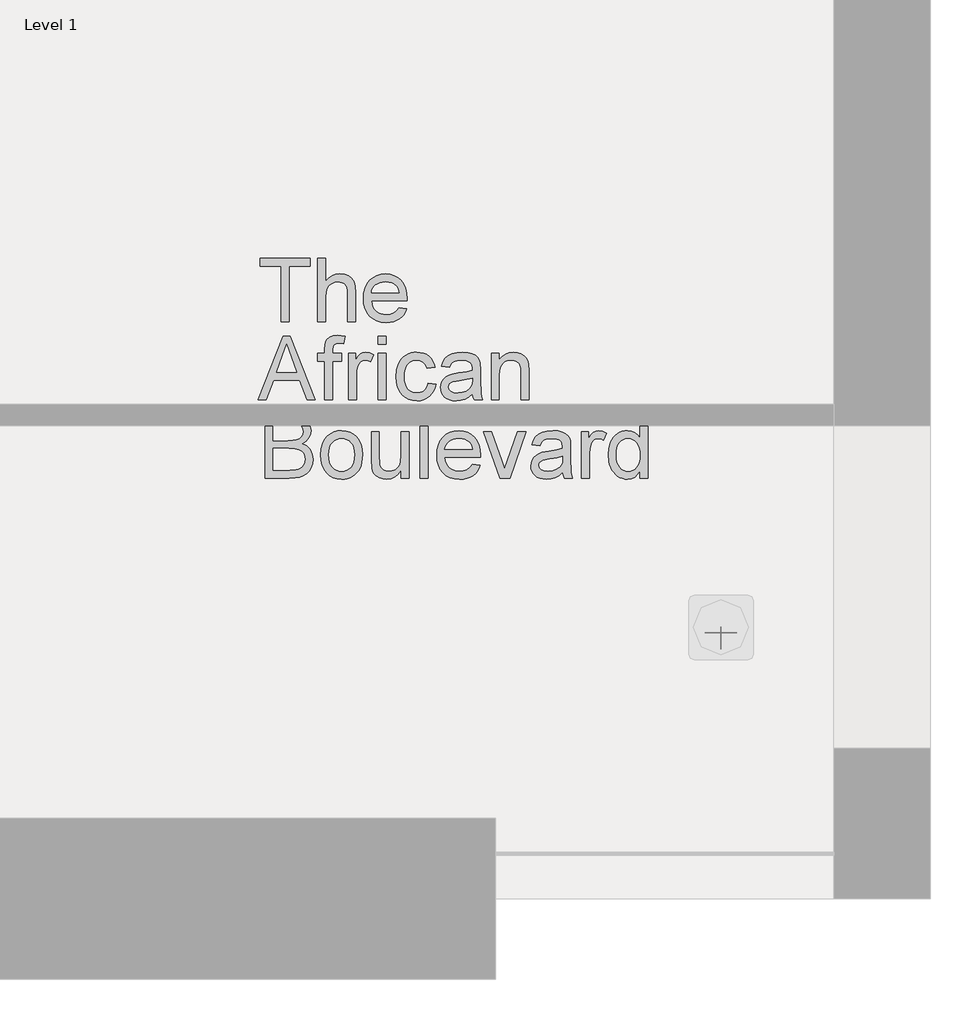
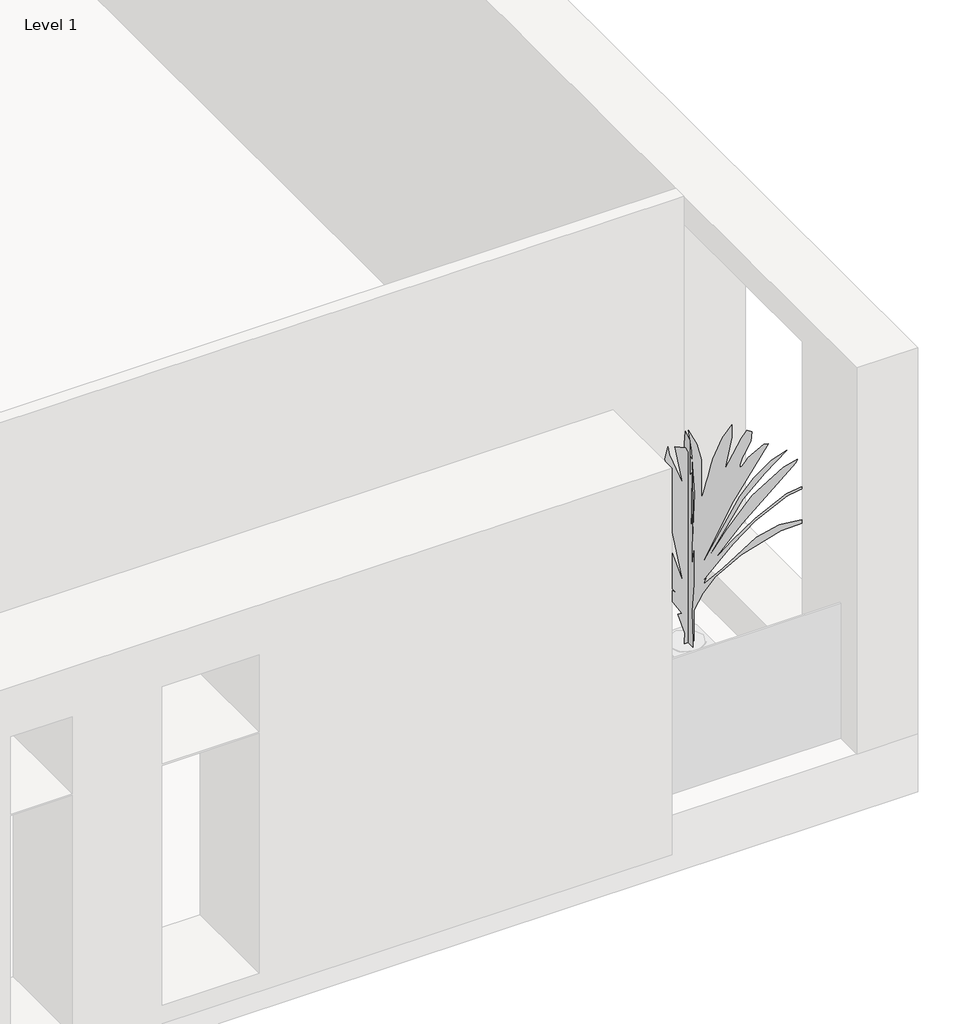
# One storey, part 3 of 3: 1 geographic element, 1 proxy.
"""IFC4 building model written with IfcOpenShell, lengths in millimetres."""

from ifc_helpers import new_model, si_unit, origin, origin_with_axes, place, context, project, spatial, polyline, outline, extrude, transform, mapped, element, save
from components import rpc_tree_tropical_0177ab4a

model = new_model("IFC4")

# Units and contexts
model_context = context("Model", 3, world=origin())
ifc_project = project(units=[si_unit("LENGTHUNIT", "METRE", prefix="MILLI")], contexts=[model_context])

# Site, building, storey
site = spatial("IfcSite", under=ifc_project)
building = spatial("IfcBuilding", under=site)
storey = spatial("IfcBuildingStorey", under=building, Name="Level 1", Elevation=0.0)

# Proxy
placement = place(None, origin())
element("IfcBuildingElementProxy", 1, Name="24\" Arial", ObjectType="24\" Arial", at=placement, inside=storey, context=model_context, shape_type="SweptSolid", body=[
    extrude(outline(polyline([(215.7046154, 0.0), (215.7046154, 525.1938462), (18.7569231, 525.1938462), (18.7569231, 600.2215385), (487.68, 600.2215385), (487.68, 525.1938462), (290.7323077, 525.1938462), (290.7323077, 0.0), (215.7046154, 0.0)])), origin_with_axes(), (0.0, 0.0, 1.0), 152.4),
    extrude(outline(polyline([(562.7076923, 0.0), (562.7076923, 600.2215385), (637.7353846, 600.2215385), (637.7353846, 379.5346154), (665.293774, 410.4359135), (696.2408654, 432.5082692), (730.5766587, 445.7516827), (768.3011538, 450.1661538), (813.6181731, 445.3487019), (852.5607692, 430.8963462), (883.2239423, 407.9447596), (903.7026923, 377.6296154), (915.2425962, 335.9760577), (919.0892308, 279.0092308), (919.0892308, 0.0), (844.0615385, 0.0), (844.0615385, 271.2426923), (842.5686779, 296.5755288), (838.0900962, 318.2082692), (830.6257933, 336.1409135), (820.1757692, 350.3734615), (806.9873077, 361.208149), (791.3076923, 368.9472115), (773.1369231, 373.590649), (752.475, 375.1384615), (720.7677404, 370.9621154), (691.0021154, 358.4330769), (666.3470192, 338.7602885), (649.9713462, 313.1526923), (640.794375, 279.1191346), (637.7353846, 234.1684615), (637.7353846, 0.0), (562.7076923, 0.0)])), origin_with_axes(), (0.0, 0.0, 1.0), 152.4),
    extrude(outline(polyline([(1330.8623077, 131.2984615), (1404.4246154, 121.92), (1393.1457332, 92.4566106), (1377.9194712, 66.4918269), (1358.7458293, 44.025649), (1335.6248077, 25.0580769), (1308.7945313, 9.9920913), (1278.493125, -0.7693269), (1244.7205889, -7.2261779), (1207.4769231, -9.3784615), (1160.9234856, -5.6646274), (1119.4439423, 5.476875), (1083.0382933, 24.0460457), (1051.7065385, 50.0428846), (1026.5110817, 82.7438582), (1008.5143269, 121.4254327), (997.716274, 166.0876082), (994.1169231, 216.7303846), (997.7529087, 269.0904087), (1008.6608654, 315.2408654), (1026.8407933, 355.1817548), (1052.2926923, 388.9130769), (1083.5420192, 415.7112981), (1119.1142308, 434.8528846), (1159.0093269, 446.3378365), (1203.2273077, 450.1661538), (1246.0211178, 446.3469952), (1284.7210096, 434.8895192), (1319.3269832, 415.793726), (1349.8390385, 389.0596154), (1374.7459976, 355.4015625), (1392.5366827, 315.5339423), (1403.2110938, 269.4567548), (1406.7692308, 217.17), (1406.3296154, 196.9476923), (1069.1446154, 196.9476923), (1073.4903966, 167.0080529), (1082.1315865, 140.7868269), (1095.0681851, 118.2840144), (1112.3001923, 99.4996154), (1132.8751082, 84.6900721), (1155.8404327, 74.1118269), (1181.1961659, 67.7648798), (1208.9423077, 65.6492308), (1248.8740385, 69.5691346), (1282.5046154, 81.3288462), (1309.8340385, 101.6610577), (1330.8623077, 131.2984615)]), holes=[polyline([(1069.1446154, 271.9753846), (1331.7415385, 271.9753846), (1321.59375, 311.6140385), (1312.8655529, 327.2020673), (1301.7011538, 339.9692308), (1281.2407212, 355.3557692), (1257.9594231, 366.3461538), (1231.8572596, 372.9403846), (1202.9342308, 375.1384615), (1176.5527284, 373.3845793), (1152.3601442, 368.1229327), (1130.3564784, 359.3535216), (1110.5417308, 347.0763462), (1093.9141947, 331.8592428), (1081.4721635, 314.2700481), (1073.215637, 294.308762), (1069.1446154, 271.9753846)])]), origin_with_axes(), (0.0, 0.0, 1.0), 152.4),
    extrude(outline(polyline([(-4.1030769, -740.8984615), (235.4873077, -140.6769231), (299.3780769, -140.6769231), (538.8219231, -740.8984615), (459.5446154, -740.8984615), (390.9646154, -553.3292308), (143.6076923, -553.3292308), (75.0276923, -740.8984615), (-4.1030769, -740.8984615)]), holes=[polyline([(171.1569231, -478.3015385), (363.5619231, -478.3015385), (309.3426923, -330.7373077), (267.2861538, -215.7046154), (229.9188462, -317.8419231), (171.1569231, -478.3015385)])]), origin_with_axes(), (0.0, 0.0, 1.0), 152.4),
    extrude(outline(polyline([(628.3569231, -740.8984615), (628.3569231, -375.1384615), (562.7076923, -375.1384615), (562.7076923, -300.1107692), (628.3569231, -300.1107692), (628.3569231, -255.7096154), (630.3351923, -218.9650962), (636.27, -193.1376923), (651.3634615, -168.1895192), (674.6630769, -148.4434615), (707.2678846, -135.5847115), (750.2769231, -131.2984615), (782.8450962, -133.35), (818.7103846, -139.5046154), (807.72, -209.8430769), (764.4911538, -206.3261538), (735.9711058, -209.4400962), (717.2325, -218.7819231), (706.8465865, -236.6229808), (703.3846154, -265.2346154), (703.3846154, -300.1107692), (787.7907692, -300.1107692), (787.7907692, -375.1384615), (703.3846154, -375.1384615), (703.3846154, -740.8984615), (628.3569231, -740.8984615)])), origin_with_axes(), (0.0, 0.0, 1.0), 152.4),
    extrude(outline(polyline([(853.44, -740.8984615), (853.44, -300.1107692), (919.0892308, -300.1107692), (919.0892308, -365.3203846), (943.3413462, -327.5134615), (965.6884615, -305.2396154), (988.1088462, -294.3591346), (1012.5807692, -290.7323077), (1049.9480769, -296.5205769), (1087.9015385, -313.8853846), (1062.8434615, -381.1465385), (1036.4665385, -369.6066346), (1010.0896154, -365.76), (987.6875481, -369.4600962), (967.6667308, -380.5603846), (951.4925481, -398.2182692), (940.6303846, -421.5911538), (931.5083654, -463.5011538), (928.4676923, -509.2211538), (928.4676923, -740.8984615), (853.44, -740.8984615)])), origin_with_axes(), (0.0, 0.0, 1.0), 152.4),
    extrude(outline(polyline([(1134.7938462, -740.8984615), (1134.7938462, -300.1107692), (1209.8215385, -300.1107692), (1209.8215385, -740.8984615), (1134.7938462, -740.8984615)])), origin_with_axes(), (0.0, 0.0, 1.0), 152.4),
    extrude(outline(polyline([(1134.7938462, -215.7046154), (1134.7938462, -140.6769231), (1209.8215385, -140.6769231), (1209.8215385, -215.7046154), (1134.7938462, -215.7046154)])), origin_with_axes(), (0.0, 0.0, 1.0), 152.4),
    extrude(outline(polyline([(1603.7169231, -581.4646154), (1678.7446154, -590.8430769), (1670.5842548, -626.2458534), (1657.82625, -657.5730288), (1640.470601, -684.8246034), (1618.5173077, -708.0005769), (1592.8913942, -726.4964784), (1564.5178846, -739.7078365), (1533.3967788, -747.6346514), (1499.5280769, -750.2769231), (1457.4486418, -746.5905649), (1419.7195673, -735.5314904), (1386.3408534, -717.0996995), (1357.3125, -691.2951923), (1333.8159736, -658.6033774), (1317.0327404, -619.5096635), (1306.9628005, -574.0140505), (1303.6061538, -522.1165385), (1309.3394712, -455.3499519), (1316.5061178, -425.304988), (1326.5394231, -397.4855769), (1339.5080769, -372.4503966), (1355.4807692, -350.758125), (1374.4575, -332.408762), (1396.4382692, -317.4023077), (1420.429363, -305.7341827), (1445.4370673, -297.3998077), (1471.4613822, -292.3991827), (1498.5023077, -290.7323077), (1531.7894351, -293.0219712), (1561.8985096, -299.8909615), (1588.8295313, -311.3392788), (1612.5825, -327.3669231), (1632.7544351, -347.6075481), (1648.9423558, -371.6948077), (1661.146262, -399.6287019), (1669.3661538, -431.4092308), (1594.3384615, -440.7876923), (1580.7287019, -408.0546635), (1559.5355769, -384.5901923), (1531.9313942, -370.4675481), (1499.0884615, -365.76), (1473.5953486, -368.0771394), (1450.6025481, -375.0285577), (1430.1100601, -386.6142548), (1412.1178846, -402.8342308), (1397.4686178, -424.0639904), (1387.0048558, -450.6790385), (1380.7265986, -482.679375), (1378.6338462, -520.065), (1380.6808053, -558.0138822), (1386.8216827, -590.3851442), (1397.0564784, -617.1787861), (1411.3851923, -638.3948077), (1429.0201803, -654.5186178), (1449.1737981, -666.035625), (1471.8460457, -672.9458293), (1497.0369231, -675.2492308), (1535.8879327, -669.4975962), (1552.6894832, -662.3080529), (1567.7417308, -652.2426923), (1580.6233774, -639.1916106), (1590.913125, -623.0449038), (1598.6109736, -603.8025721), (1603.7169231, -581.4646154)])), origin_with_axes(), (0.0, 0.0, 1.0), 152.4),
    extrude(outline(polyline([(2025.7476923, -684.6276923), (1989.9007212, -715.3641346), (1952.9913462, -735.4765385), (1914.1769712, -746.5768269), (1872.615, -750.2769231), (1839.2088101, -748.0513702), (1809.9148558, -741.3747115), (1784.733137, -730.2469471), (1763.6636538, -714.6680769), (1747.0269591, -695.6272356), (1735.1436058, -674.1135577), (1728.0135938, -650.1270433), (1725.6369231, -623.6676923), (1729.2271154, -592.5649038), (1739.9976923, -564.3196154), (1756.6114904, -540.1407692), (1777.7313462, -521.2373077), (1802.5512981, -506.9498077), (1830.2653846, -496.6188462), (1895.1819231, -485.3353846), (1971.8948077, -473.4657692), (2025.3080769, -459.5446154), (2025.7476923, -442.8392308), (2020.5822115, -409.3551923), (2014.1253606, -396.954375), (2005.0857692, -387.4476923), (1989.4611058, -377.9593269), (1970.4294231, -371.1819231), (1922.145, -365.76), (1877.4507692, -369.3685096), (1846.2380769, -380.1940385), (1824.9533654, -400.2148558), (1810.0430769, -431.4092308), (1735.0153846, -422.0307692), (1748.0389904, -381.0), (1767.4736538, -348.7615385), (1795.1327885, -324.1064423), (1832.8298077, -305.8257692), (1878.9344712, -294.5056731), (1931.8165385, -290.7323077), (1982.5371635, -294.0660577), (2022.7436538, -304.0673077), (2053.0587981, -319.1058173), (2074.1053846, -337.5513462), (2088.0631731, -360.3563942), (2097.1119231, -388.4734615), (2100.7753846, -454.1226923), (2100.7753846, -547.4676923), (2104.5853846, -677.8136538), (2110.2271154, -710.0337981), (2119.5323077, -740.8984615), (2044.5046154, -740.8984615), (2032.4884615, -714.8146154), (2025.7476923, -684.6276923)]), holes=[polyline([(2025.7476923, -534.5723077), (1975.3384615, -547.0647115), (1904.7069231, -557.5788462), (1840.1567308, -569.7415385), (1823.3597596, -578.0575962), (1810.9223077, -589.5242308), (1803.2290385, -603.2622115), (1800.6646154, -618.3923077), (1806.2513942, -640.7027885), (1823.0117308, -658.9834615), (1850.5792788, -671.1827885), (1888.5876923, -675.2492308), (1928.8857692, -670.7614904), (1964.4946154, -657.2982692), (1993.3626923, -637.460625), (2013.4384615, -613.8496154), (2022.3406731, -589.5242308), (2025.3080769, -555.8203846), (2025.7476923, -534.5723077)])]), origin_with_axes(), (0.0, 0.0, 1.0), 152.4),
    extrude(outline(polyline([(2203.9384615, -740.8984615), (2203.9384615, -300.1107692), (2278.9661538, -300.1107692), (2278.9661538, -361.6569231), (2305.0316827, -330.6274038), (2336.3359615, -308.4634615), (2372.8789904, -295.1650962), (2414.6607692, -290.7323077), (2451.6434135, -294.3041827), (2485.5121154, -305.0198077), (2513.7574038, -321.5420192), (2533.8698077, -342.5336538), (2547.5162019, -367.9397596), (2556.3634615, -397.7053846), (2560.32, -470.2419231), (2560.32, -740.8984615), (2485.2923077, -740.8984615), (2485.2923077, -480.3530769), (2483.1308654, -441.5570192), (2476.6465385, -413.9711538), (2464.6853365, -394.2067788), (2446.0932692, -378.8751923), (2422.2624519, -369.0387981), (2394.585, -365.76), (2371.8028486, -367.6008894), (2350.6417788, -373.1235577), (2331.1017909, -382.3280048), (2313.1828846, -395.2142308), (2298.2130649, -413.2476202), (2287.5203365, -437.8935577), (2281.1046995, -469.1520433), (2278.9661538, -507.0230769), (2278.9661538, -740.8984615), (2203.9384615, -740.8984615)])), origin_with_axes(), (0.0, 0.0, 1.0), 152.4),
    extrude(outline(polyline([(65.6492308, -1481.7969231), (65.6492308, -881.5753846), (294.6888462, -881.5753846), (357.6820673, -885.9898558), (406.8640385, -899.2332692), (426.8573798, -909.2482572), (444.5610577, -921.6353365), (459.9750721, -936.3945072), (473.0994231, -953.5257692), (491.0687019, -991.0396154), (497.0584615, -1030.3119231), (492.0212019, -1066.4519712), (476.9094231, -1100.4305769), (451.6132212, -1130.1595673), (416.0226923, -1153.5507692), (438.6674639, -1163.2039904), (458.5371635, -1175.7513462), (475.6317909, -1191.1928365), (489.9513462, -1209.5284615), (501.266863, -1230.1995433), (509.349375, -1252.6474038), (514.1988822, -1276.8720433), (515.8153846, -1302.8734615), (511.4009135, -1344.7285096), (498.1575, -1383.5428846), (478.393125, -1416.5506731), (454.4157692, -1440.9859615), (425.053125, -1458.6804808), (389.1328846, -1471.4659615), (345.4827404, -1479.2141827), (292.9303846, -1481.7969231), (65.6492308, -1481.7969231)]), holes=[polyline([(140.6769231, -1125.4153846), (277.6903846, -1125.4153846), (325.6084615, -1123.8034615), (357.7003846, -1118.9676923), (385.7075481, -1107.8490865), (405.8382692, -1091.1986538), (417.9826442, -1069.2728365), (422.0307692, -1042.3280769), (418.2574038, -1016.1709615), (406.9373077, -993.3842308), (388.5833654, -975.598125), (363.7084615, -964.4428846), (325.5351923, -958.5630288), (267.2861538, -956.6030769), (140.6769231, -956.6030769), (140.6769231, -1125.4153846)]), polyline([(140.6769231, -1406.7692308), (294.5423077, -1406.7692308), (350.2269231, -1403.8384615), (376.0726442, -1397.3358173), (397.3390385, -1387.4994231), (414.6305769, -1373.4134135), (428.5517308, -1354.1619231), (437.7287019, -1330.6058654), (440.7876923, -1303.6061538), (437.1975, -1272.2469231), (426.4269231, -1245.2838462), (407.6150481, -1224.200625), (379.9009615, -1210.4809615), (340.6469712, -1202.9525481), (287.2153846, -1200.4430769), (140.6769231, -1200.4430769), (140.6769231, -1406.7692308)])]), origin_with_axes(), (0.0, 0.0, 1.0), 152.4),
    extrude(outline(polyline([(590.8430769, -1261.4030769), (594.9003606, -1204.3171875), (607.0722115, -1155.1260577), (627.3586298, -1113.8296875), (655.7596154, -1080.4280769), (684.3529327, -1059.0792548), (715.9136538, -1043.8300962), (750.4417788, -1034.680601), (787.9373077, -1031.6307692), (829.3298438, -1035.3446034), (866.7566827, -1046.4861058), (900.2178245, -1065.0552764), (929.7132692, -1091.0521154), (953.7867909, -1123.5973918), (970.9821635, -1161.811875), (981.299387, -1205.6955649), (984.7384615, -1255.2484615), (983.218125, -1295.4091587), (978.6571154, -1331.0454808), (971.0554327, -1362.1574279), (960.4130769, -1388.745), (946.8628486, -1411.7103245), (930.5375481, -1431.9555288), (911.4371755, -1449.480613), (889.5617308, -1464.2855769), (865.7629688, -1476.0498678), (840.8926442, -1484.4529327), (814.9507572, -1489.4947716), (787.9373077, -1491.1753846), (745.9403005, -1487.4752885), (708.1654327, -1476.375), (674.6127043, -1457.8745192), (645.2821154, -1431.9738462), (621.4650361, -1399.1125962), (604.4528365, -1359.7303846), (594.2455168, -1313.8272115), (590.8430769, -1261.4030769)]), holes=[polyline([(665.8707692, -1261.2565385), (668.0413702, -1297.6484495), (674.5531731, -1329.1587981), (685.4061779, -1355.7875841), (700.6003846, -1377.5348077), (719.0825481, -1394.4279447), (739.7994231, -1406.4944712), (762.7510096, -1413.734387), (787.9373077, -1416.1476923), (812.9953846, -1413.720649), (835.8553846, -1406.4395192), (856.5173077, -1394.3043029), (874.9811538, -1377.315), (890.1753606, -1355.3525481), (901.0283654, -1328.2978846), (907.5401683, -1296.1510096), (909.7107692, -1258.9119231), (907.5264303, -1223.6740024), (900.9734135, -1192.9879327), (890.0517188, -1166.8537139), (874.7613462, -1145.2713462), (856.2288101, -1128.3782091), (835.580625, -1116.3116827), (812.8167909, -1109.0717668), (787.9373077, -1106.6584615), (762.7510096, -1109.0626082), (739.7994231, -1116.2750481), (719.0825481, -1128.2957813), (700.6003846, -1145.1248077), (685.4061779, -1166.8079207), (674.5531731, -1193.3909135), (668.0413702, -1224.8737861), (665.8707692, -1261.2565385)])]), origin_with_axes(), (0.0, 0.0, 1.0), 152.4),
    extrude(outline(polyline([(1350.4984615, -1481.7969231), (1350.4984615, -1406.0365385), (1323.3522115, -1443.2847837), (1291.7365385, -1469.8906731), (1255.6514423, -1485.8542067), (1215.0969231, -1491.1753846), (1178.5538942, -1487.4386538), (1144.5386538, -1476.2284615), (1116.0002885, -1459.3765385), (1095.8878846, -1438.7146154), (1082.3513942, -1413.6199038), (1073.5407692, -1383.4696154), (1069.1446154, -1313.7173077), (1069.1446154, -1041.0092308), (1144.1723077, -1041.0092308), (1144.1723077, -1278.4015385), (1145.3079808, -1325.88), (1148.715, -1354.8946154), (1159.6504327, -1380.410625), (1178.3890385, -1399.8086538), (1203.6852404, -1412.0629327), (1234.2934615, -1416.1476923), (1266.6601442, -1411.9713462), (1296.9386538, -1399.4423077), (1321.9051442, -1379.7145673), (1338.3357692, -1353.9421154), (1347.4577885, -1318.6446635), (1350.4984615, -1270.3419231), (1350.4984615, -1041.0092308), (1425.5261538, -1041.0092308), (1425.5261538, -1481.7969231), (1350.4984615, -1481.7969231)])), origin_with_axes(), (0.0, 0.0, 1.0), 152.4),
    extrude(outline(polyline([(1528.6892308, -1481.7969231), (1528.6892308, -881.5753846), (1603.7169231, -881.5753846), (1603.7169231, -1481.7969231), (1528.6892308, -1481.7969231)])), origin_with_axes(), (0.0, 0.0, 1.0), 152.4),
    extrude(outline(polyline([(2024.8684615, -1350.4984615), (2098.4307692, -1359.8769231), (2087.151887, -1389.3403125), (2071.925625, -1415.3050962), (2052.7519832, -1437.771274), (2029.6309615, -1456.7388462), (2002.8006851, -1471.8048317), (1972.4992788, -1482.56625), (1938.7267428, -1489.023101), (1901.4830769, -1491.1753846), (1854.9296394, -1487.4615505), (1813.4500962, -1476.3200481), (1777.0444471, -1457.7508774), (1745.7126923, -1431.7540385), (1720.5172356, -1399.0530649), (1702.5204808, -1360.3714904), (1691.7224279, -1315.7093149), (1688.1230769, -1265.0665385), (1691.7590625, -1212.7065144), (1702.6670192, -1166.5560577), (1720.8469471, -1126.6151683), (1746.2988462, -1092.8838462), (1777.5481731, -1066.085625), (1813.1203846, -1046.9440385), (1853.0154808, -1035.4590865), (1897.2334615, -1031.6307692), (1940.0272716, -1035.4499279), (1978.7271635, -1046.9074038), (2013.333137, -1066.0031971), (2043.8451923, -1092.7373077), (2068.7521514, -1126.3953606), (2086.5428365, -1166.2629808), (2097.2172476, -1212.3401683), (2100.7753846, -1264.6269231), (2100.3357692, -1284.8492308), (1763.1507692, -1284.8492308), (1767.4965505, -1314.7888702), (1776.1377404, -1341.0100962), (1789.0743389, -1363.5129087), (1806.3063462, -1382.2973077), (1826.881262, -1397.106851), (1849.8465865, -1407.6850962), (1875.2023197, -1414.0320433), (1902.9484615, -1416.1476923), (1942.8801923, -1412.2277885), (1976.5107692, -1400.4680769), (2003.8401923, -1380.1358654), (2024.8684615, -1350.4984615)]), holes=[polyline([(1763.1507692, -1209.8215385), (2025.7476923, -1209.8215385), (2015.5999038, -1170.1828846), (2006.8717067, -1154.5948558), (1995.7073077, -1141.8276923), (1975.246875, -1126.4411538), (1951.9655769, -1115.4507692), (1925.8634135, -1108.8565385), (1896.9403846, -1106.6584615), (1870.5588822, -1108.4123437), (1846.3662981, -1113.6739904), (1824.3626322, -1122.4434014), (1804.5478846, -1134.7205769), (1787.9203486, -1149.9376803), (1775.4783173, -1167.526875), (1767.2217909, -1187.4881611), (1763.1507692, -1209.8215385)])]), origin_with_axes(), (0.0, 0.0, 1.0), 152.4),
    extrude(outline(polyline([(2284.2415385, -1481.7969231), (2128.9107692, -1041.0092308), (2208.1880769, -1041.0092308), (2302.2657692, -1305.0715385), (2330.5476923, -1393.8738462), (2358.2434615, -1310.0538462), (2452.7607692, -1041.0092308), (2532.1846154, -1041.0092308), (2379.0519231, -1481.7969231), (2284.2415385, -1481.7969231)])), origin_with_axes(), (0.0, 0.0, 1.0), 152.4),
    extrude(outline(polyline([(2879.1876923, -1425.5261538), (2843.3407212, -1456.2625962), (2806.4313462, -1476.375), (2767.6169712, -1487.4752885), (2726.055, -1491.1753846), (2692.6488101, -1488.9498317), (2663.3548558, -1482.2731731), (2638.173137, -1471.1454087), (2617.1036538, -1455.5665385), (2600.4669591, -1436.5256971), (2588.5836058, -1415.0120192), (2581.4535937, -1391.0255048), (2579.0769231, -1364.5661538), (2582.6671154, -1333.4633654), (2593.4376923, -1305.2180769), (2610.0514904, -1281.0392308), (2631.1713462, -1262.1357692), (2655.9912981, -1247.8482692), (2683.7053846, -1237.5173077), (2748.6219231, -1226.2338462), (2825.3348077, -1214.3642308), (2878.7480769, -1200.4430769), (2879.1876923, -1183.7376923), (2874.0222115, -1150.2536538), (2867.5653606, -1137.8528365), (2858.5257692, -1128.3461538), (2842.9011058, -1118.8577885), (2823.8694231, -1112.0803846), (2775.585, -1106.6584615), (2730.8907692, -1110.2669712), (2699.6780769, -1121.0925), (2678.3933654, -1141.1133173), (2663.4830769, -1172.3076923), (2588.4553846, -1162.9292308), (2601.4789904, -1121.8984615), (2620.9136538, -1089.66), (2648.5727885, -1065.0049038), (2686.2698077, -1046.7242308), (2732.3744712, -1035.4041346), (2785.2565385, -1031.6307692), (2835.9771635, -1034.9645192), (2876.1836538, -1044.9657692), (2906.4987981, -1060.0042788), (2927.5453846, -1078.4498077), (2941.5031731, -1101.2548558), (2950.5519231, -1129.3719231), (2954.2153846, -1195.0211538), (2954.2153846, -1288.3661538), (2958.0253846, -1418.7121154), (2963.6671154, -1450.9322596), (2972.9723077, -1481.7969231), (2897.9446154, -1481.7969231), (2885.9284615, -1455.7130769), (2879.1876923, -1425.5261538)]), holes=[polyline([(2879.1876923, -1275.4707692), (2828.7784615, -1287.9631731), (2758.1469231, -1298.4773077), (2693.5967308, -1310.64), (2676.7997596, -1318.9560577), (2664.3623077, -1330.4226923), (2656.6690385, -1344.1606731), (2654.1046154, -1359.2907692), (2659.6913942, -1381.60125), (2676.4517308, -1399.8819231), (2704.0192788, -1412.08125), (2742.0276923, -1416.1476923), (2782.3257692, -1411.6599519), (2817.9346154, -1398.1967308), (2846.8026923, -1378.3590865), (2866.8784615, -1354.7480769), (2875.7806731, -1330.4226923), (2878.7480769, -1296.7188462), (2879.1876923, -1275.4707692)])]), origin_with_axes(), (0.0, 0.0, 1.0), 152.4),
    extrude(outline(polyline([(3057.3784615, -1481.7969231), (3057.3784615, -1041.0092308), (3123.0276923, -1041.0092308), (3123.0276923, -1106.2188462), (3147.2798077, -1068.4119231), (3169.6269231, -1046.1380769), (3192.0473077, -1035.2575962), (3216.5192308, -1031.6307692), (3253.8865385, -1037.4190385), (3291.84, -1054.7838462), (3266.7819231, -1122.045), (3240.405, -1110.5050962), (3214.0280769, -1106.6584615), (3191.6260096, -1110.3585577), (3171.6051923, -1121.4588462), (3155.4310096, -1139.1167308), (3144.5688462, -1162.4896154), (3135.4468269, -1204.3996154), (3132.4061538, -1250.1196154), (3132.4061538, -1481.7969231), (3057.3784615, -1481.7969231)])), origin_with_axes(), (0.0, 0.0, 1.0), 152.4),
    extrude(outline(polyline([(3610.7076923, -1481.7969231), (3610.7076923, -1411.0188462), (3588.2598317, -1446.0873317), (3561.0677885, -1471.13625), (3529.1315625, -1486.165601), (3492.4511538, -1491.1753846), (3467.6861538, -1489.3619712), (3443.9469231, -1483.9217308), (3421.2334615, -1474.8546635), (3399.5457692, -1462.1607692), (3379.5615865, -1446.2201322), (3361.9586538, -1427.4128365), (3346.7369712, -1405.7388822), (3333.8965385, -1381.1982692), (3323.7029567, -1354.2580889), (3316.4218269, -1325.3854327), (3310.5969231, -1261.8426923), (3315.9638942, -1199.0875962), (3332.0648077, -1142.4138462), (3344.1359135, -1117.1634375), (3358.8813462, -1095.0452885), (3376.3011058, -1076.059399), (3396.3951923, -1060.2057692), (3418.4538101, -1047.7042067), (3441.7671635, -1038.7745192), (3466.3352524, -1033.4167067), (3492.1580769, -1031.6307692), (3528.8659615, -1036.7412981), (3561.3242308, -1052.0728846), (3588.8368269, -1075.5739904), (3610.7076923, -1105.1930769), (3610.7076923, -881.5753846), (3685.7353846, -881.5753846), (3685.7353846, -1481.7969231), (3610.7076923, -1481.7969231)]), holes=[polyline([(3385.6246154, -1261.5496154), (3387.7402644, -1297.9323678), (3394.0872115, -1329.4152404), (3404.6654567, -1355.9982332), (3419.475, -1377.6813462), (3437.1603606, -1394.5103726), (3456.3660577, -1406.5311058), (3477.0920913, -1413.7435457), (3499.3384615, -1416.1476923), (3521.6901563, -1413.8534495), (3542.2925481, -1406.9707212), (3561.145637, -1395.4995072), (3578.2494231, -1379.4398077), (3592.4499159, -1358.6634014), (3602.593125, -1333.0420673), (3608.6790505, -1302.5758053), (3610.7076923, -1267.2646154), (3608.6424159, -1228.5509856), (3602.4465865, -1195.3508654), (3592.1202043, -1167.6642548), (3577.6632692, -1145.4911538), (3560.1839784, -1128.501851), (3540.7905288, -1116.3666346), (3519.4829207, -1109.0855048), (3496.2611538, -1106.6584615), (3473.5751683, -1108.9893389), (3452.8491346, -1115.9819712), (3434.0830529, -1127.6363582), (3417.2769231, -1143.9525), (3403.4290385, -1165.2875841), (3393.5376923, -1191.9987981), (3387.6028846, -1224.0861418), (3385.6246154, -1261.5496154)])]), origin_with_axes(), (0.0, 0.0, 1.0), 152.4),
])

# Geographic element
rpc_tree_tropical_shape = rpc_tree_tropical_0177ab4a(model_context)
element("IfcGeographicElement", 2, ObjectType="RPC Tree - Tropical", at=placement, inside=storey, context=model_context, shape_type="MappedRepresentation", body=[
    mapped(rpc_tree_tropical_shape, transform((4377.8125281, -2943.3632813, 0.0), x_axis=(1.0, 0.0, 0.0), y_axis=(0.0, 1.0, 0.0), z_axis=(0.0, 0.0, 1.0))),
])

save(model, "model.ifc")

# Revit data of these elements
# Type "RPC Tree - Tropical"
#   built-in parameter 1005198 = "{2, 15},{39, RPC-16-G2M6-EAFX-C5H6-W000-ST1L-LVER-AU},{1, 0},{1, 0},{2, 13},{1, 8},{5, Color},{1, 0},{1, 0},{3, 0.8},{3, 0.8},{3, 0.8},{1, 8},{7, BBoxMin},{1, 0},{1, 0},{1, 0},{1, 0},{1, 0},{1, 8},{7, BBoxMax},{1, 0},{1, 0},{1, 0},{1, 0},{1, 0},{2, 11},{9, RPCTypeId},{1, 0},{1, 0},{39, RPC-16-G2M6-EAFX-C5H6-W000-ST1L-LVER-AU},{1, 6},{14, RPCPlantHeight},{1, 0},{1, 0},{2, 13},{2, 11},{7, keyword},{1, 0},{1, 0},{35, :RPCs:Trees [Tropical]:Geometry:RPC},{2, 11},{8, category},{1, 0},{1, 0},{16, Trees [Tropical]},{2, 11},{12, LocalizedUID},{1, 0},{1, 0},{15, Traveler's Palm},{2, 14},{6, Height},{1, 0},{1, 0},{2, 13},{1, 2},{16, Cast Reflections},{1, 0},{1, 0},{1, 0},{1, 2},{12, Cast Shadows},{1, 0},{1, 0},{1, 1},{1, 2},{9, Lock View},{1, 0},{1, 0},{1, 0},{1, 4},{5, ViewC},{1, 0},{1, 0},{1, 0},{21, assetlibrary_base.fbx},{1, 5},"
#   built-in parameter 1005195 = "RPC-16-G2M6-EAFX-C5H6-W000-ST1L-LVER-AU"
#   Assembly Code = "G2050500"
#   Height = 13' - 0"
#   Plan Symbol = element 321958
#   Default Elevation = 0
# Element 1 (IfcBuildingElementProxy, "24\" Arial")
#   Phase Created = New Construction
# Element 2 (IfcGeographicElement, "RPC Tree - Tropical")
#   Phase Created = New Construction
